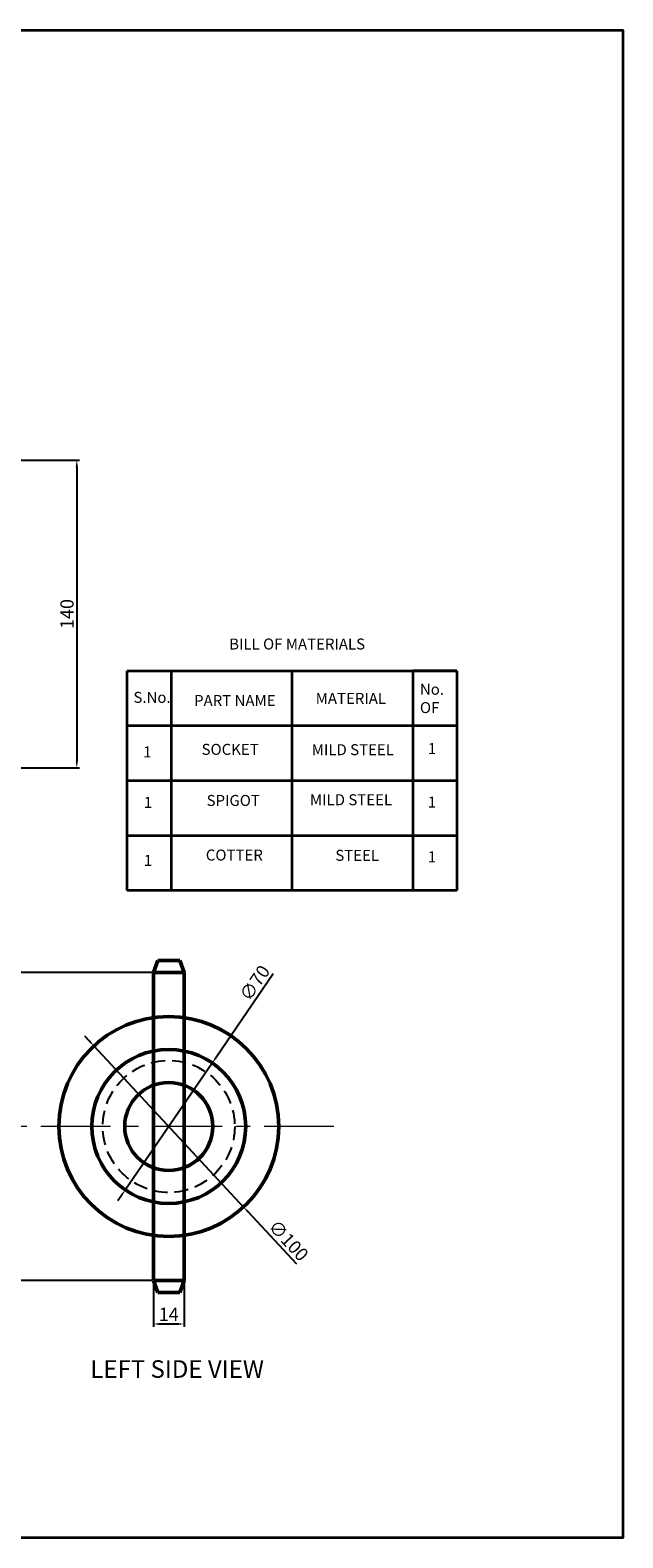
# Model space of a CAD drawing. Units: millimetres. Extents: x 641 to 1388, y -43 to 643.
# Tile 3 of 3: x 1119 to 1388, y -43 to 643. Entities that reach past the tile are written whole.
import ezdxf

# ---------------------------------------------------------------- set-up
doc = ezdxf.new("R2010")
doc.units = ezdxf.units.MM
doc.linetypes.add('CENTER', pattern=[50.8, 31.75, -6.35, 6.35, -6.35])
doc.linetypes.add('HIDDEN', pattern=[9.525, 6.35, -3.175])
for name, color, linetype, lineweight in [('M-CNTR', 1, 'CENTER', 18), ('M-DIMS', 2, 'Continuous', 25), ('M-HIDN', 4, 'HIDDEN', 25), ('M-OUTL', 7, 'Continuous', 50), ('M-TEXT', 3, 'Continuous', 25), ('M-TTLB', 7, 'Continuous', 35)]:
    doc.layers.add(name, color=color, linetype=linetype, lineweight=lineweight)
doc.styles.get("Standard").update_dxf_attribs({"font": 'arial.ttf'})
doc.dimstyles.new('ISO-25', dxfattribs={"dimtxt": 6, "dimasz": 3, "dimexe": 1.25, "dimexo": 0.625, "dimtad": 1, "dimdec": 0, "dimtxsty": 'Standard', "dimcen": 2.5, "dimadec": 0, "dimazin": 0, "dimtfac": 1, "dimtdec": 0, "dimtmove": 0, "dimatfit": 3, "dimfxl": 1, "dimarcsym": 0})

# ---------------------------------------------------------------- blocks, each defined once
blk = doc.blocks.new('*D9')
at = {"layer": 'Defpoints', "color": 0, "transparency": 16777216}
for p in [(1107.03, 447.38), (1107.03, 307.38), (1140.01, 307.38)]:
    blk.add_point(p, dxfattribs=at)
at = {"layer": 'M-DIMS', "color": 0, "lineweight": -2, "transparency": 16777216}
for p, q in [((1107.65, 447.38), (1141.26, 447.38)), ((1140.01, 444.38), (1140.01, 310.38)), ((1107.65, 307.38), (1141.26, 307.38))]:
    blk.add_line(p, q, dxfattribs=at)
at = {"layer": 'M-DIMS', "color": 0, "transparency": 16777216}
for points in [[(1139.51, 444.38), (1140.51, 444.38), (1140.01, 447.38)], [(1139.51, 310.38), (1140.51, 310.38), (1140.01, 307.38)]]:
    blk.add_solid(points, dxfattribs=at)
at = {"layer": 'M-DIMS', "color": 0, "transparency": 16777216, "insert": (1136.32, 377.38), "char_height": 6, "attachment_point": 5, "rotation": 90}
blk.add_mtext('140', dxfattribs=at)
blk = doc.blocks.new('*D26')
at = {"layer": 'Defpoints', "color": 0, "transparency": 16777216}
for p in [(1174.83, 214.4), (1114.12, 74.4), (1174.83, 74.4)]:
    blk.add_point(p, dxfattribs=at)
at = {"layer": 'M-DIMS', "color": 0, "lineweight": -2, "transparency": 16777216}
for p, q in [((1174.21, 214.4), (1112.87, 214.4)), ((1114.12, 211.4), (1114.12, 77.4)), ((1174.21, 74.4), (1112.87, 74.4))]:
    blk.add_line(p, q, dxfattribs=at)
at = {"layer": 'M-DIMS', "color": 0, "transparency": 16777216}
for points in [[(1113.62, 211.4), (1114.62, 211.4), (1114.12, 214.4)], [(1113.62, 77.4), (1114.62, 77.4), (1114.12, 74.4)]]:
    blk.add_solid(points, dxfattribs=at)
at = {"layer": 'M-DIMS', "color": 0, "transparency": 16777216, "insert": (1110.43, 144.4), "char_height": 6, "attachment_point": 5, "rotation": 90}
blk.add_mtext('140', dxfattribs=at)
blk = doc.blocks.new('*D27')
at = {"layer": 'Defpoints', "color": 0, "transparency": 16777216}
for p in [(1201.63, 173.26), (1162.04, 115.53)]:
    blk.add_point(p, dxfattribs=at)
at = {"layer": 'M-DIMS', "color": 0, "lineweight": -2, "transparency": 16777216}
for p, q in [((1229.4, 213.75), (1203.33, 175.73)), ((1162.04, 115.53), (1201.63, 173.26)), ((1160.34, 113.06), (1158.64, 110.58))]:
    blk.add_line(p, q, dxfattribs=at)
at = {"layer": 'M-DIMS', "color": 0, "transparency": 16777216}
for points in [[(1202.91, 176.02), (1203.74, 175.45), (1201.63, 173.26)], [(1159.93, 113.34), (1160.75, 112.78), (1162.04, 115.53)]]:
    blk.add_solid(points, dxfattribs=at)
at = {"layer": 'M-DIMS', "color": 0, "transparency": 16777216, "insert": (1221.59, 209.19), "char_height": 6, "attachment_point": 5, "rotation": 55.55512}
blk.add_mtext('∅70', dxfattribs=at)
blk = doc.blocks.new('*D28')
at = {"layer": 'Defpoints', "color": 0, "transparency": 16777216}
for p in [(1147.8, 181.02), (1215.87, 107.77)]:
    blk.add_point(p, dxfattribs=at)
at = {"layer": 'M-DIMS', "color": 0, "lineweight": -2, "transparency": 16777216}
for p, q in [((1145.75, 183.22), (1143.71, 185.42)), ((1147.8, 181.02), (1215.87, 107.77)), ((1240.08, 81.71), (1217.91, 105.57))]:
    blk.add_line(p, q, dxfattribs=at)
at = {"layer": 'M-DIMS', "color": 0, "transparency": 16777216}
for points in [[(1146.12, 183.56), (1145.39, 182.88), (1147.8, 181.02)], [(1218.28, 105.91), (1217.54, 105.23), (1215.87, 107.77)]]:
    blk.add_solid(points, dxfattribs=at)
at = {"layer": 'M-DIMS', "color": 0, "transparency": 16777216, "insert": (1235.75, 92.03), "char_height": 6, "attachment_point": 5, "rotation": 312.90064}
blk.add_mtext('∅100', dxfattribs=at)
blk = doc.blocks.new('*D29')
at = {"layer": 'Defpoints', "color": 0, "transparency": 16777216}
for p in [(1174.83, 81.18), (1188.83, 81.18), (1188.83, 54.58)]:
    blk.add_point(p, dxfattribs=at)
at = {"layer": 'M-DIMS', "color": 0, "lineweight": -2, "transparency": 16777216}
for p, q in [((1174.83, 80.55), (1174.83, 53.33)), ((1188.83, 80.55), (1188.83, 53.33)), ((1177.83, 54.58), (1185.83, 54.58))]:
    blk.add_line(p, q, dxfattribs=at)
at = {"layer": 'M-DIMS', "color": 0, "transparency": 16777216}
for points in [[(1177.83, 55.08), (1177.83, 54.08), (1174.83, 54.58)], [(1185.83, 55.08), (1185.83, 54.08), (1188.83, 54.58)]]:
    blk.add_solid(points, dxfattribs=at)
at = {"layer": 'M-DIMS', "color": 0, "transparency": 16777216, "insert": (1181.83, 58.21), "char_height": 6, "attachment_point": 5}
blk.add_mtext('14', dxfattribs=at)

msp = doc.modelspace()

# ---------------------------------------------------------------- linework, layer by layer
at = {"layer": 'M-CNTR'}
msp.add_line((1256.973, 144.396), (794.875, 144.396), dxfattribs=at)
at = {"layer": 'M-HIDN'}
msp.add_circle((1181.832, 144.396), 30, dxfattribs=at)
at = {"layer": 'M-OUTL'}
for p, q in [((1176.832, 219.866), (1174.832, 214.396)), ((1186.832, 219.866), (1176.832, 219.866)), ((1186.832, 219.866), (1188.832, 214.396)), ((1174.832, 214.396), (1174.832, 74.396)), ((1188.832, 214.396), (1174.832, 214.396)), ((1188.832, 74.396), (1188.832, 214.396)), ((1174.832, 74.396), (1188.832, 74.396)), ((1176.832, 68.926), (1174.832, 74.396)), ((1186.832, 68.926), (1176.832, 68.926)), ((1186.832, 68.926), (1188.832, 74.396))]:
    msp.add_line(p, q, dxfattribs=at)
for radius in [50, 35, 20]:
    msp.add_circle((1181.832, 144.396), radius, dxfattribs=at)
at = {"layer": 'M-TTLB'}
for p, q in [((1162.895, 351.622), (1312.895, 351.622)), ((1162.895, 251.622), (1162.895, 351.622)), ((1182.895, 351.622), (1182.895, 251.622)), ((1237.895, 351.622), (1237.895, 251.622)), ((1312.895, 351.622), (1292.895, 351.622)), ((1292.895, 351.622), (1292.895, 251.622)), ((1312.895, 351.622), (1312.895, 251.622)), ((1162.895, 326.622), (1312.895, 326.622)), ((1162.895, 301.622), (1312.895, 301.622)), ((1162.895, 276.622), (1312.895, 276.622)), ((1312.895, 251.622), (1162.895, 251.622))]:
    msp.add_line(p, q, dxfattribs=at)
msp.add_lwpolyline([(641.348, 642.837), (1388.388, 642.837), (1388.388, -42.647), (641.348, -42.647)], close=True, dxfattribs=at)

# ---------------------------------------------------------------- texts
at = {"layer": 'M-TEXT', "attachment_point": 1}
for s, width, insert, char_height in [('\\pxqc;BILL OF MATERIALS', 129.07358, (1175.683, 366.241), 5), ('No. OF', 14.82427, (1296.075, 345.663), 5), ('S.No.', 14.82427, (1165.762, 341.986), 5), ('\\pxqc;PART NAME', 39.87563, (1191.954, 340.554), 5), ('\\pxqc;MATERIAL', 39.87563, (1244.731, 341.503), 5), ('\\pxqc;1', 5, (1169.573, 317.203), 5), ('\\pxqc;SOCKET', 44.18575, (1187.676, 318.329), 5), ('\\pxqc;MILD STEEL', 44.18575, (1243.469, 318.193), 5), ('\\pxqc;1', 5, (1299.04, 318.696), 5), ('\\pxqc;SPIGOT', 36.2377, (1193.055, 295.108), 5), ('\\pxqc;MILD STEEL', 41.29437, (1244.095, 295.434), 5), ('\\pxqc;1', 5, (1169.891, 294.243), 5), ('\\pxqc;1', 5, (1299.04, 294.377), 5), ('\\pxqc;1', 5, (1169.891, 267.875), 5), ('\\pxqc;COTTER', 36.26953, (1193.522, 270.295), 5), ('\\pxqc;STEEL', 41.6829, (1246.708, 270.16), 5), ('\\pxqc;1', 5, (1299.04, 269.49), 5), ('\\pxqc;LEFT SIDE VIEW', 131.26047, (1120.022, 38.097), 8)]:
    msp.add_mtext_dynamic_manual_height_columns(s, width=width, gutter_width=12.5, heights=[0], dxfattribs=dict(at, insert=insert, char_height=char_height))

# ---------------------------------------------------------------- dimensions: what is measured, and where the dimension line sits
at = {"layer": 'M-DIMS'}
for base, p1, p2, picture, middle in [((1140.008, 307.376), (1107.03, 447.376), (1107.03, 307.376), '*D9', (1136.319, 377.376)), ((1114.115, 74.396), (1174.832, 214.396), (1174.832, 74.396), '*D26', (1110.427, 144.396))]:
    dim = msp.add_linear_dim(base=base, p1=p1, p2=p2, angle=90, dimstyle='ISO-25', override={"dimclrd": 0, "dimclre": 0, "dimclrt": 0}, dxfattribs=at)
    dim.commit()
    dim.dimension.update_dxf_attribs({"geometry": picture, "text_midpoint": middle})
for p1, p2, picture, middle in [((1162.036, 115.532), (1201.628, 173.259), '*D27', (1224.775, 207.007)), ((1147.796, 181.023), (1215.868, 107.769), '*D28', (1232.93, 89.41))]:
    dim = msp.add_diameter_dim_2p(p1=p1, p2=p2, dimstyle='ISO-25', override={"dimclrd": 0, "dimclre": 0, "dimclrt": 0}, dxfattribs=at)
    dim.commit()
    dim.dimension.update_dxf_attribs({"geometry": picture, "text_midpoint": middle, "dimtype": 163})
dim = msp.add_linear_dim(base=(1188.832, 54.578), p1=(1174.832, 81.179), p2=(1188.832, 81.179), dimstyle='ISO-25', override={"dimclrd": 0, "dimclre": 0, "dimclrt": 0}, dxfattribs=at)
dim.commit()
dim.dimension.update_dxf_attribs({"geometry": '*D29', "text_midpoint": (1181.832, 58.215)})

doc.saveas('drawing.dxf')
